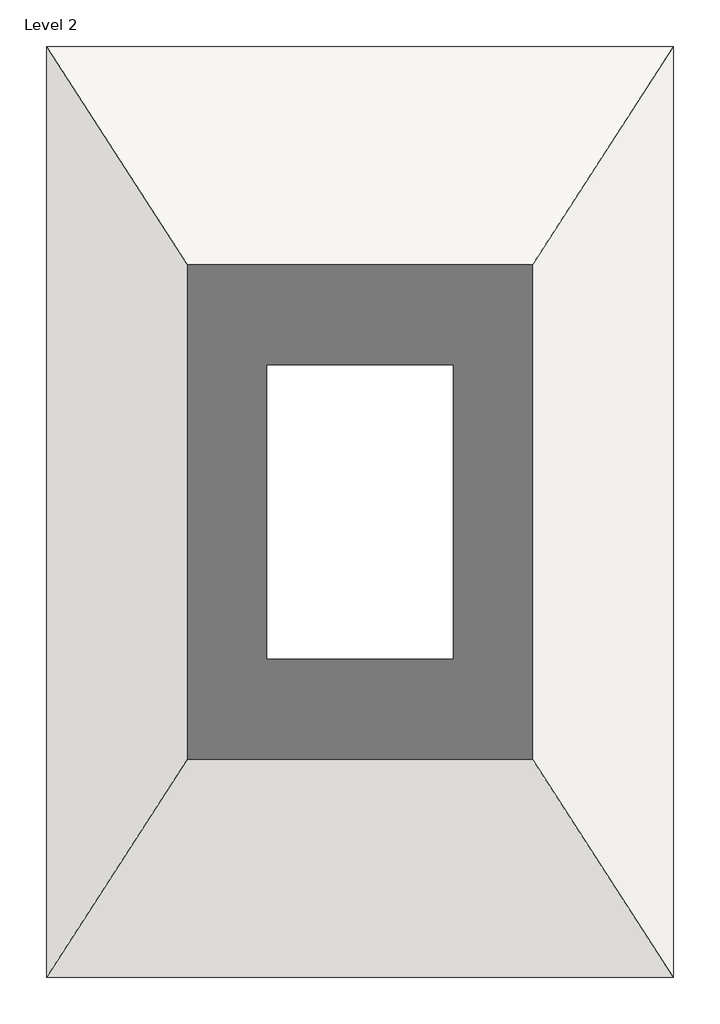
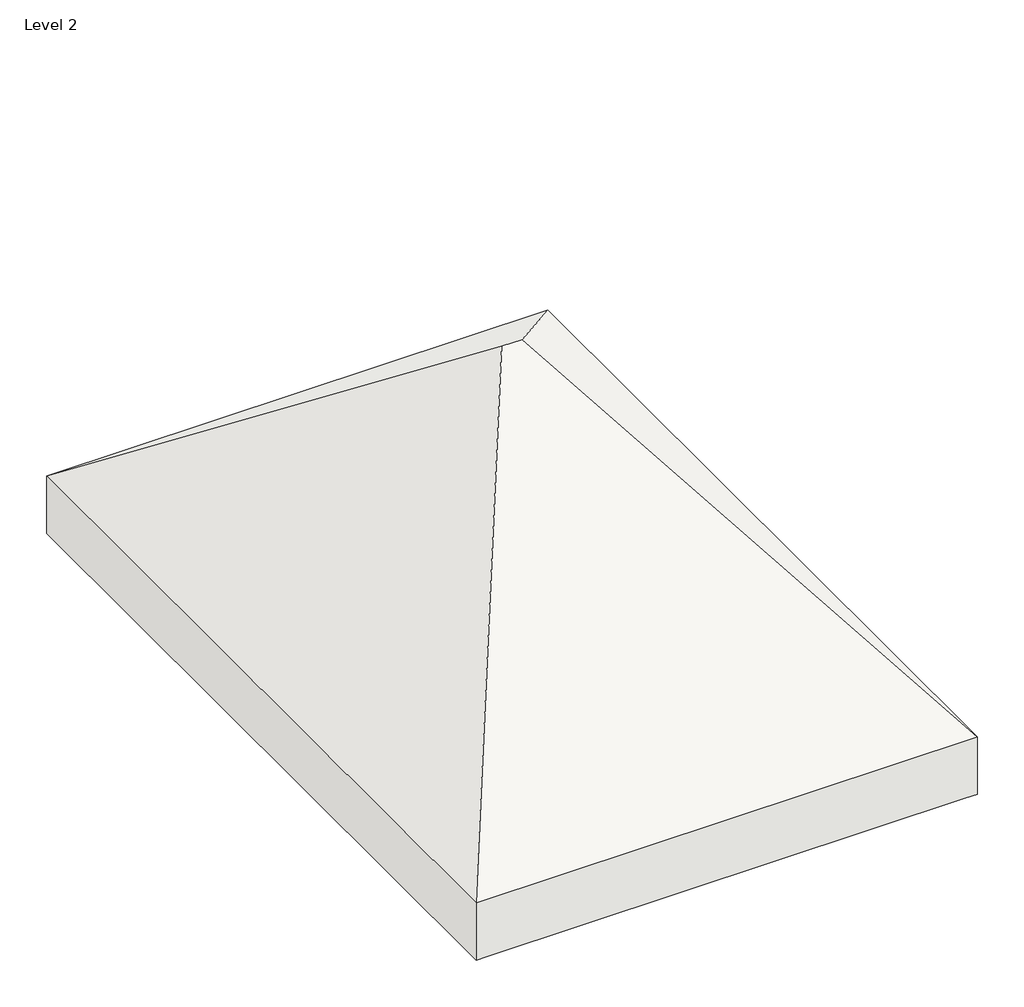
# One storey: 1 roof.
"""IFC4 building model written with IfcOpenShell, lengths in millimetres."""

from ifc_helpers import new_model, si_unit, origin, place, context, project, spatial, faceted_brep, element, save

model = new_model("IFC4")

# Units and contexts
model_context = context("Model", 3, world=origin())
ifc_project = project(units=[si_unit("LENGTHUNIT", "METRE", prefix="MILLI")], contexts=[model_context])

# Site, building, storey
site = spatial("IfcSite", under=ifc_project)
building = spatial("IfcBuilding", under=site)
storey = spatial("IfcBuildingStorey", under=building, Name="Level 2", Elevation=3048.0)

# Roof
placement = place(None, origin())
element("IfcRoof", 1, ObjectType="Generic - 12\"", at=placement, inside=storey, context=model_context, shape_type="Brep", body=[
    faceted_brep([(-7848.8563022, 12444.4599287, 3048.0), (-9349.6289971, 10122.5025247, 4789.468053), (-10850.401692, 12444.4599287, 3048.0), (-9349.6289971, 10092.8173326, 4789.468053), (-10850.401692, 7770.8599287, 3048.0), (-7848.8563022, 7770.8599287, 3048.0), (-7774.8289971, 12444.4599287, 3429.0), (-10924.4289971, 12444.4599287, 3429.0), (-9414.0629466, 10107.6599287, 5181.6), (-9285.1950475, 10107.6599287, 5181.6), (-10924.4289971, 7770.8599287, 3429.0), (-7774.8289971, 7770.8599287, 3429.0), (-10924.4289971, 12444.4599287, 3048.0), (-7774.8289971, 12444.4599287, 3048.0), (-10924.4289971, 7770.8599287, 3048.0), (-7774.8289971, 7770.8599287, 3048.0)], [[[0, 1, 2]], [[2, 1, 3, 4]], [[4, 3, 5]], [[1, 0, 5, 3]], [[6, 7, 8, 9]], [[7, 10, 8]], [[10, 11, 9, 8]], [[6, 9, 11]], [[12, 7, 6, 13, 0, 2]], [[14, 10, 7, 12]], [[15, 11, 10, 14, 4, 5]], [[13, 6, 11, 15]], [[13, 15, 5, 0]], [[4, 14, 12, 2]]]),
])

save(model, "model.ifc")

# Revit data of these elements
# Type "Generic - 12\""
#   Assembly Code = "B1020"
#   Layers, outside or top first: 1' - 0" "roof" (function 1)
# Element 1 (IfcRoof, "Generic - 12\"")
#   built-in parameter 1001705 = 17 (stored number, unit not read)
#   built-in parameter 1001710 = 33615
#   Phase Created = New Construction
#   Materials on its faces: "roof"
# Materials
#   "roof": class "Generic", colour RGB 120 120 120, transparency 0, Cost = 0
